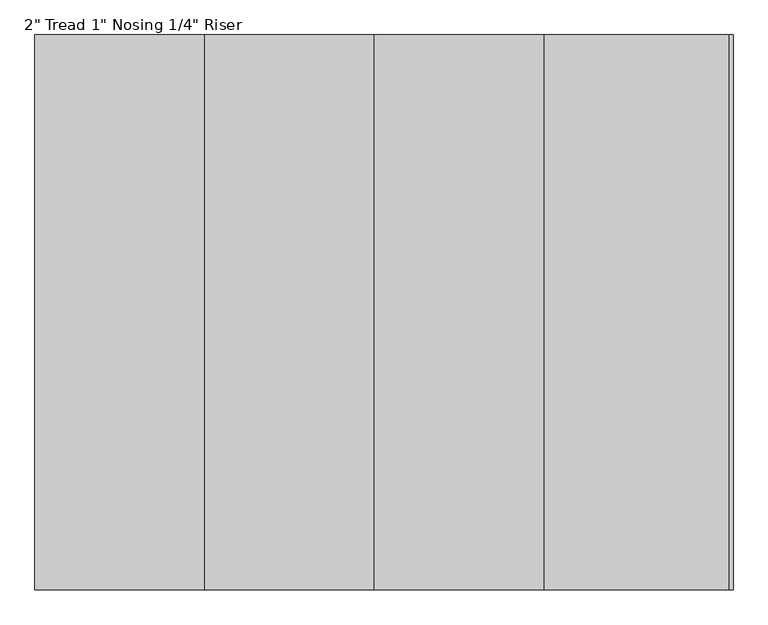
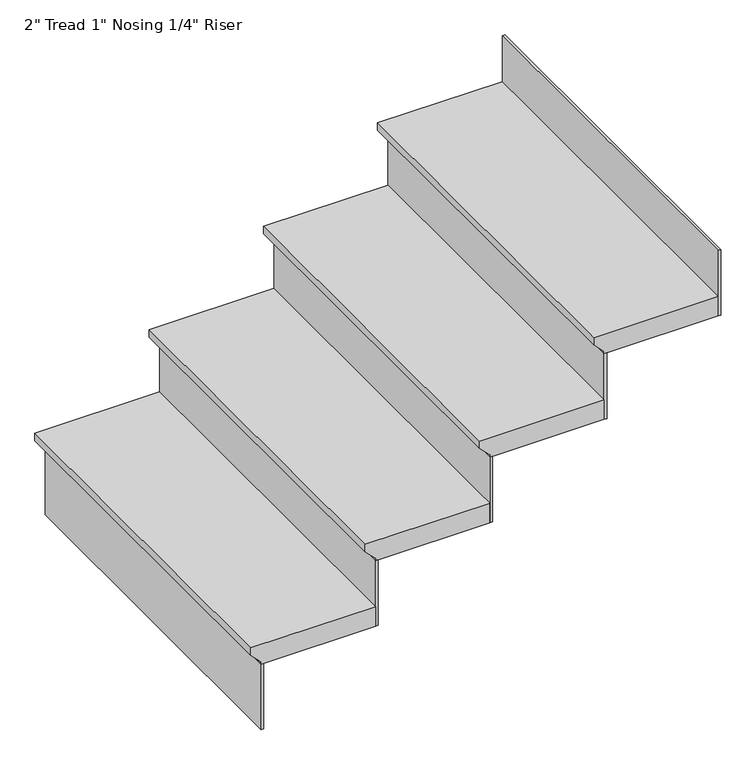
"""IFC4 building model written with IfcOpenShell, lengths in millimetres: stair flight geometry."""

from ifc_helpers import new_model, si_unit, frame, origin, place, context, project, spatial, polyline, outline, extrude, source, transform, mapped, element, save


def stair_flight_1517cfd2(model_context):
    return source(origin(), model_context, "Body", "SweptSolid", [
        extrude(outline(polyline([(2370.6666667, -7535.6823175), (2370.6666667, -7840.4823175), (2351.6166667, -7840.4823175), (2326.2166667, -7815.0823175), (2319.8666667, -7815.0823175), (2319.8666667, -7535.6823175), (2370.6666667, -7535.6823175)])), frame((0.0, 7352.205876, 0.0), z_axis=(0.0, 1.0, 0.0), x_axis=(0.0, 0.0, 1.0)), (0.0, 0.0, 1.0), 914.4),
        extrude(outline(polyline([(-7808.7323175, 7352.205876), (-7815.0823175, 7352.205876), (-7815.0823175, 8266.605876), (-7808.7323175, 8266.605876), (-7808.7323175, 7352.205876)])), frame((0.0, 0.0, 2150.5333333), z_axis=(0.0, 0.0, 1.0), x_axis=(1.0, 0.0, 0.0)), (0.0, 0.0, 1.0), 169.3333333),
        extrude(outline(polyline([(-7529.3323175, 7352.205876), (-7535.6823175, 7352.205876), (-7535.6823175, 8266.605876), (-7529.3323175, 8266.605876), (-7529.3323175, 7352.205876)])), frame((0.0, 0.0, 2319.8666667), z_axis=(0.0, 0.0, 1.0), x_axis=(1.0, 0.0, 0.0)), (0.0, 0.0, 1.0), 169.3333333),
        extrude(outline(polyline([(2540.0, -7256.2823175), (2540.0, -7561.0823175), (2520.95, -7561.0823175), (2495.55, -7535.6823175), (2489.2, -7535.6823175), (2489.2, -7256.2823175), (2540.0, -7256.2823175)])), frame((0.0, 7352.205876, 0.0), z_axis=(0.0, 1.0, 0.0), x_axis=(0.0, 0.0, 1.0)), (0.0, 0.0, 1.0), 914.4),
        extrude(outline(polyline([(-7249.9323175, 7352.205876), (-7256.2823175, 7352.205876), (-7256.2823175, 8266.605876), (-7249.9323175, 8266.605876), (-7249.9323175, 7352.205876)])), frame((0.0, 0.0, 2489.2), z_axis=(0.0, 0.0, 1.0), x_axis=(1.0, 0.0, 0.0)), (0.0, 0.0, 1.0), 169.3333333),
        extrude(outline(polyline([(2709.3333333, -6976.8823175), (2709.3333333, -7281.6823175), (2690.2833333, -7281.6823175), (2664.8833333, -7256.2823175), (2658.5333333, -7256.2823175), (2658.5333333, -6976.8823175), (2709.3333333, -6976.8823175)])), frame((0.0, 7352.205876, 0.0), z_axis=(0.0, 1.0, 0.0), x_axis=(0.0, 0.0, 1.0)), (0.0, 0.0, 1.0), 914.4),
        extrude(outline(polyline([(-6970.5323175, 7352.205876), (-6976.8823175, 7352.205876), (-6976.8823175, 8266.605876), (-6970.5323175, 8266.605876), (-6970.5323175, 7352.205876)])), frame((0.0, 0.0, 2658.5333333), z_axis=(0.0, 0.0, 1.0), x_axis=(1.0, 0.0, 0.0)), (0.0, 0.0, 1.0), 169.3333333),
        extrude(outline(polyline([(-6691.1323175, 7352.205876), (-6697.4823175, 7352.205876), (-6697.4823175, 8266.605876), (-6691.1323175, 8266.605876), (-6691.1323175, 7352.205876)])), frame((0.0, 0.0, 2827.8666667), z_axis=(0.0, 0.0, 1.0), x_axis=(1.0, 0.0, 0.0)), (0.0, 0.0, 1.0), 169.3333333),
        extrude(outline(polyline([(2878.6666667, -6697.4823175), (2878.6666667, -7002.2823175), (2859.6166667, -7002.2823175), (2834.2166667, -6976.8823175), (2827.8666667, -6976.8823175), (2827.8666667, -6697.4823175), (2878.6666667, -6697.4823175)])), frame((0.0, 7352.205876, 0.0), z_axis=(0.0, 1.0, 0.0), x_axis=(0.0, 0.0, 1.0)), (0.0, 0.0, 1.0), 914.4),
    ])


if __name__ == "__main__":
    model = new_model("IFC4")
    model_context = context("Model", 3, world=origin())
    ifc_project = project(units=[si_unit("LENGTHUNIT", "METRE", prefix="MILLI")], contexts=[model_context])
    site = spatial("IfcSite", under=ifc_project)
    building = spatial("IfcBuilding", under=site)
    placement = place(None, origin())
    stair_flight_shape = stair_flight_1517cfd2(model_context)
    element("IfcStairFlight", 1, ObjectType="2\" Tread 1\" Nosing 1/4\" Riser", at=placement, inside=building, context=model_context, shape_type="MappedRepresentation", body=[
        mapped(stair_flight_shape, transform((0.0, 0.0, 0.0), x_axis=(1.0, 0.0, 0.0), y_axis=(0.0, 1.0, 0.0), z_axis=(0.0, 0.0, 1.0))),
    ])
    save(model, "model.ifc")
